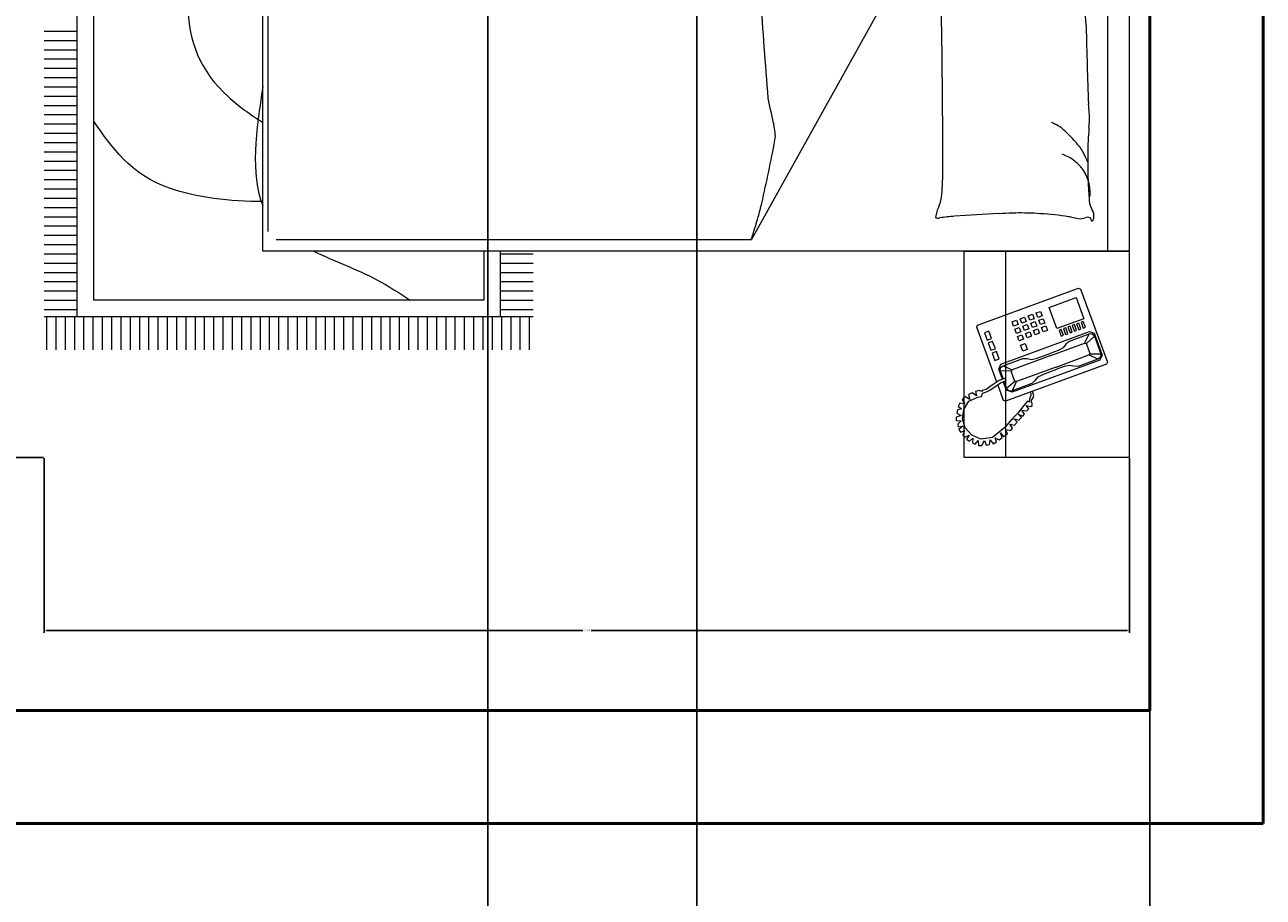
# Model space of a CAD drawing. Units: inches. Extents: x 338 to 1188, y -996 to 127.
# Tile 10 of 15: x 859 to 957, y -622 to -552. Entities that reach past the tile are written whole.
import ezdxf

# ---------------------------------------------------------------- set-up
doc = ezdxf.new("R2010")
doc.units = ezdxf.units.IN
doc.header["$MEASUREMENT"] = 0
doc.layers.add('A-ANNO-DIMS', color=5, linetype='Continuous', lineweight=18)
doc.layers.add('wall', color=1, linetype='Continuous', lineweight=50)
doc.layers.add('furniture', color=50, linetype='Continuous', lineweight=13, transparency=0.8)
doc.styles.add('DIM_FONT', font='SIMPLEX.shx', dxfattribs={"width": 0.8})
doc.styles.get("Standard").update_dxf_attribs({"font": 'arial.ttf'})
doc.dimstyles.get("Standard").update_dxf_attribs({"dimtxt": 0.18, "dimasz": 0.18, "dimexe": 0.18, "dimexo": 0.0625, "dimgap": 0.09, "dimtad": 0, "dimtih": 1, "dimtoh": 1, "dimdec": 1, "dimzin": 0, "dimdsep": 46, "dimlunit": 4, "dimtxsty": 'Standard', "dimcen": 0.09, "dimadec": 0, "dimazin": 0, "dimtfac": 1, "dimtdec": 1, "dimtofl": 0, "dimtmove": 0, "dimatfit": 3, "dimfxl": 1, "dimtolj": 1, "dimtzin": 0, "dimarcsym": 0})

# ---------------------------------------------------------------- blocks, each defined once
blk = doc.blocks.new('A$C4F634EDD')
for p, q in [((0.5, 2.6295), (2.3, 2.6295)), ((2.3, 2.6295), (2.3, 0.5295)), ((2.3, 2.6295), (2.8, 2.6295)), ((2.3, 2.2295), (2.3, 2.6295)), ((2.8, 2.6295), (2.8, 2.2295)), ((0.5, 2.5771), (2.3, 2.5771)), ((2.392, 2.5115), (2.5692, 2.5765)), ((2.4985, 2.5445), (2.5516, 2.564)), ((2.5062, 2.5454), (2.5487, 2.561)), ((2.5483, 2.5347), (2.5487, 2.561)), ((2.5487, 2.561), (2.5571, 2.56)), ((2.5615, 2.5536), (2.5514, 2.5318)), ((2.5516, 2.564), (2.5637, 2.5584)), ((2.5571, 2.56), (2.5615, 2.5536)), ((2.5615, 2.5536), (2.5791, 2.5058)), ((2.5637, 2.5584), (2.6418, 2.3458)), ((2.5692, 2.5765), (2.574, 2.5743)), ((2.574, 2.5743), (2.6638, 2.3298)), ((2.4842, 2.5232), (2.47, 2.518)), ((2.4862, 2.5179), (2.4842, 2.5232)), ((2.4946, 2.5331), (2.4985, 2.5445)), ((2.5734, 2.3187), (2.4946, 2.5331)), ((2.5062, 2.5454), (2.5004, 2.5392)), ((2.5004, 2.5392), (2.5013, 2.5315)), ((2.5013, 2.5315), (2.5188, 2.4836)), ((2.5013, 2.5315), (2.5231, 2.5214)), ((2.5235, 2.5256), (2.5062, 2.5454)), ((2.5231, 2.5214), (2.5235, 2.5256)), ((2.5483, 2.5347), (2.5235, 2.5256)), ((2.5514, 2.5318), (2.5483, 2.5347)), ((2.5807, 2.4521), (2.5514, 2.5318)), ((2.3898, 2.5066), (2.392, 2.5115)), ((2.4795, 2.2621), (2.3898, 2.5066)), ((2.412, 2.5007), (2.4634, 2.5196)), ((2.4361, 2.4352), (2.412, 2.5007)), ((2.4634, 2.5196), (2.4875, 2.454)), ((2.47, 2.518), (2.472, 2.5127)), ((2.472, 2.5127), (2.4862, 2.5179)), ((2.4881, 2.5126), (2.4739, 2.5074)), ((2.4739, 2.5074), (2.4759, 2.502)), ((2.4759, 2.502), (2.4901, 2.5073)), ((2.492, 2.5019), (2.4778, 2.4967)), ((2.4778, 2.4967), (2.4798, 2.4914)), ((2.4798, 2.4914), (2.494, 2.4966)), ((2.4901, 2.5073), (2.4881, 2.5126)), ((2.494, 2.4966), (2.492, 2.5019)), ((2.5523, 2.4417), (2.5231, 2.5214)), ((2.5788, 2.4956), (2.5767, 2.4848)), ((2.5791, 2.5058), (2.5788, 2.4956)), ((2.4959, 2.4913), (2.4817, 2.4861)), ((2.4817, 2.4861), (2.4837, 2.4808)), ((2.4837, 2.4808), (2.4979, 2.486)), ((2.4998, 2.4807), (2.4856, 2.4755)), ((2.4856, 2.4755), (2.4876, 2.4702)), ((2.4876, 2.4702), (2.5018, 2.4754)), ((2.5037, 2.47), (2.4895, 2.4648)), ((2.4895, 2.4648), (2.4915, 2.4595)), ((2.4915, 2.4595), (2.5057, 2.4647)), ((2.4979, 2.486), (2.4959, 2.4913)), ((2.5018, 2.4754), (2.4998, 2.4807)), ((2.5057, 2.4647), (2.5037, 2.47)), ((2.5188, 2.4836), (2.5256, 2.4761)), ((2.5256, 2.4761), (2.5342, 2.4692)), ((2.5342, 2.4692), (2.5405, 2.4574)), ((2.5767, 2.4848), (2.5795, 2.4717)), ((2.5795, 2.4717), (2.586, 2.454)), ((2.4875, 2.454), (2.4361, 2.4352)), ((2.4811, 2.4276), (2.4917, 2.4315)), ((2.4917, 2.4315), (2.4956, 2.4208)), ((2.5405, 2.4574), (2.547, 2.4397)), ((2.5594, 2.4061), (2.547, 2.4397)), ((2.5523, 2.4417), (2.5875, 2.346)), ((2.5807, 2.4521), (2.6158, 2.3564)), ((2.5984, 2.4204), (2.586, 2.454)), ((2.4457, 2.4146), (2.4563, 2.4185)), ((2.4496, 2.4039), (2.4457, 2.4146)), ((2.4602, 2.4078), (2.4496, 2.4039)), ((2.4563, 2.4185), (2.4602, 2.4078)), ((2.4634, 2.4211), (2.474, 2.425)), ((2.4673, 2.4104), (2.4634, 2.4211)), ((2.4779, 2.4143), (2.4673, 2.4104)), ((2.4706, 2.4016), (2.4812, 2.4055)), ((2.4745, 2.3909), (2.4706, 2.4016)), ((2.474, 2.425), (2.4779, 2.4143)), ((2.485, 2.4169), (2.4811, 2.4276)), ((2.4812, 2.4055), (2.4851, 2.3949)), ((2.4956, 2.4208), (2.485, 2.4169)), ((2.4883, 2.4081), (2.4989, 2.412)), ((2.4922, 2.3975), (2.4883, 2.4081)), ((2.5028, 2.4014), (2.4922, 2.3975)), ((2.4989, 2.412), (2.5028, 2.4014)), ((2.5622, 2.393), (2.5594, 2.4061)), ((2.6047, 2.4086), (2.5984, 2.4204)), ((2.6133, 2.4017), (2.6047, 2.4086)), ((2.6201, 2.3941), (2.6133, 2.4017)), ((2.4528, 2.3951), (2.4635, 2.399)), ((2.4567, 2.3844), (2.4528, 2.3951)), ((2.4674, 2.3883), (2.4567, 2.3844)), ((2.46, 2.3756), (2.4706, 2.3795)), ((2.4639, 2.365), (2.46, 2.3756)), ((2.4635, 2.399), (2.4674, 2.3883)), ((2.4706, 2.3795), (2.4745, 2.3689)), ((2.4851, 2.3949), (2.4745, 2.3909)), ((2.4777, 2.3821), (2.4883, 2.386)), ((2.4816, 2.3715), (2.4777, 2.3821)), ((2.4922, 2.3754), (2.4816, 2.3715)), ((2.4883, 2.386), (2.4922, 2.3754)), ((2.4954, 2.3886), (2.5061, 2.3925)), ((2.4993, 2.378), (2.4954, 2.3886)), ((2.51, 2.3819), (2.4993, 2.378)), ((2.5026, 2.3691), (2.5132, 2.373)), ((2.5061, 2.3925), (2.51, 2.3819)), ((2.5132, 2.373), (2.5171, 2.3624)), ((2.5238, 2.3769), (2.538, 2.3821)), ((2.5277, 2.3663), (2.5238, 2.3769)), ((2.5419, 2.3715), (2.5277, 2.3663)), ((2.538, 2.3821), (2.5419, 2.3715)), ((2.5598, 2.372), (2.5601, 2.3822)), ((2.5774, 2.3242), (2.5598, 2.372)), ((2.5601, 2.3822), (2.5622, 2.393)), ((2.6376, 2.3463), (2.6201, 2.3941)), ((2.6499, 2.3979), (2.6397, 2.3953)), ((2.6417, 2.39), (2.6488, 2.391)), ((2.6488, 2.391), (2.6538, 2.3895)), ((2.6551, 2.397), (2.6499, 2.3979)), ((2.6538, 2.3895), (2.6596, 2.388)), ((2.6627, 2.392), (2.6551, 2.397)), ((2.6596, 2.388), (2.6626, 2.3867)), ((2.6626, 2.3867), (2.6662, 2.388)), ((2.6692, 2.394), (2.6627, 2.392)), ((2.6662, 2.388), (2.6632, 2.3828)), ((2.6632, 2.3828), (2.6736, 2.3744)), ((2.6736, 2.3944), (2.6692, 2.394)), ((2.6765, 2.391), (2.6736, 2.3944)), ((2.6736, 2.3744), (2.6922, 2.3593)), ((2.6742, 2.3795), (2.6765, 2.391)), ((2.6824, 2.3858), (2.6742, 2.3795)), ((2.6873, 2.3815), (2.6824, 2.3858)), ((2.6853, 2.369), (2.6873, 2.3815)), ((2.6946, 2.376), (2.6853, 2.369)), ((2.6995, 2.3713), (2.6946, 2.376)), ((2.695, 2.3603), (2.6995, 2.3713)), ((2.4745, 2.3689), (2.4639, 2.365)), ((2.4672, 2.3561), (2.4778, 2.36)), ((2.4711, 2.3455), (2.4672, 2.3561)), ((2.4817, 2.3494), (2.4711, 2.3455)), ((2.4778, 2.36), (2.4817, 2.3494)), ((2.4849, 2.3626), (2.4955, 2.3665)), ((2.4888, 2.352), (2.4849, 2.3626)), ((2.4994, 2.3559), (2.4888, 2.352)), ((2.4955, 2.3665), (2.4994, 2.3559)), ((2.5065, 2.3585), (2.5026, 2.3691)), ((2.5171, 2.3624), (2.5065, 2.3585)), ((2.5774, 2.3242), (2.5875, 2.346)), ((2.5875, 2.346), (2.5905, 2.3431)), ((2.5905, 2.3431), (2.5901, 2.3168)), ((2.6154, 2.3522), (2.5905, 2.3431)), ((2.6158, 2.3564), (2.6154, 2.3522)), ((2.6154, 2.3522), (2.6327, 2.3324)), ((2.6376, 2.3463), (2.6158, 2.3564)), ((2.6418, 2.3458), (2.6369, 2.332)), ((2.6385, 2.3386), (2.6376, 2.3463)), ((2.6922, 2.3593), (2.7051, 2.3473)), ((2.7031, 2.3682), (2.695, 2.3603)), ((2.7096, 2.3616), (2.7031, 2.3682)), ((2.7051, 2.3473), (2.7079, 2.3475)), ((2.7062, 2.351), (2.7096, 2.3616)), ((2.7147, 2.3578), (2.7062, 2.351)), ((2.7079, 2.3475), (2.7079, 2.3443)), ((2.7079, 2.3443), (2.727, 2.3277)), ((2.7214, 2.3517), (2.7147, 2.3578)), ((2.7196, 2.34), (2.7214, 2.3517)), ((2.7286, 2.3466), (2.7196, 2.34)), ((2.7346, 2.3423), (2.7286, 2.3466)), ((2.732, 2.3295), (2.7346, 2.3423)), ((2.8, 2.3301), (2.3, 2.3301)), ((2.561, 2.3141), (2.5433, 2.3076)), ((2.5649, 2.3035), (2.561, 2.3141)), ((2.5855, 2.3131), (2.5734, 2.3187)), ((2.5818, 2.3178), (2.5774, 2.3242)), ((2.5901, 2.3168), (2.5818, 2.3178)), ((2.6104, 2.3222), (2.5855, 2.3131)), ((2.5901, 2.3168), (2.6097, 2.324)), ((2.613, 2.3312), (2.6077, 2.3293)), ((2.6077, 2.3293), (2.6135, 2.3141)), ((2.6192, 2.3174), (2.613, 2.3312)), ((2.6135, 2.3141), (2.6244, 2.2977)), ((2.6153, 2.3261), (2.6327, 2.3324)), ((2.6369, 2.332), (2.6161, 2.3243)), ((2.626, 2.3069), (2.6192, 2.3174)), ((2.6616, 2.3249), (2.6234, 2.3109)), ((2.6327, 2.3324), (2.6385, 2.3386)), ((2.6638, 2.3298), (2.6616, 2.3249)), ((2.727, 2.3277), (2.7512, 2.2983)), ((2.7423, 2.3345), (2.732, 2.3295)), ((2.7406, 2.3172), (2.7495, 2.325)), ((2.7519, 2.3218), (2.7406, 2.3172)), ((2.7495, 2.325), (2.7423, 2.3345)), ((2.7575, 2.3144), (2.7519, 2.3218)), ((2.7526, 2.3045), (2.7575, 2.3144)), ((2.6172, 2.3086), (2.4844, 2.2599)), ((2.5114, 2.2959), (2.4936, 2.2894)), ((2.4936, 2.2894), (2.4976, 2.2788)), ((2.4976, 2.2788), (2.5153, 2.2853)), ((2.5153, 2.2853), (2.5114, 2.2959)), ((2.5362, 2.305), (2.5185, 2.2985)), ((2.5185, 2.2985), (2.5224, 2.2879)), ((2.5224, 2.2879), (2.5401, 2.2944)), ((2.5401, 2.2944), (2.5362, 2.305)), ((2.5433, 2.3076), (2.5472, 2.297)), ((2.5472, 2.297), (2.5649, 2.3035)), ((2.6244, 2.2977), (2.6349, 2.2825)), ((2.6365, 2.2916), (2.626, 2.3069)), ((2.6349, 2.2825), (2.638, 2.273)), ((2.6407, 2.2834), (2.6365, 2.2916)), ((2.6438, 2.2739), (2.6407, 2.2834)), ((2.7512, 2.2983), (2.756, 2.2695)), ((2.7622, 2.308), (2.7526, 2.3045)), ((2.7574, 2.2924), (2.7673, 2.2997)), ((2.7687, 2.2905), (2.7574, 2.2924)), ((2.7587, 2.279), (2.7699, 2.2828)), ((2.7673, 2.2997), (2.7622, 2.308)), ((2.7699, 2.2828), (2.7687, 2.2905)), ((2.4844, 2.2599), (2.4795, 2.2621)), ((2.6399, 2.2712), (2.6374, 2.2659)), ((2.6374, 2.2659), (2.6398, 2.257)), ((2.638, 2.273), (2.6399, 2.2712)), ((2.6398, 2.257), (2.6509, 2.259)), ((2.6509, 2.259), (2.6431, 2.2492)), ((2.6519, 2.2716), (2.6438, 2.2739)), ((2.6535, 2.2628), (2.6519, 2.2716)), ((2.6636, 2.2409), (2.6535, 2.2628)), ((2.756, 2.2695), (2.7459, 2.2483)), ((2.7708, 2.2725), (2.7587, 2.279)), ((2.759, 2.2637), (2.7706, 2.2643)), ((2.7676, 2.2559), (2.759, 2.2637)), ((2.7645, 2.2498), (2.7676, 2.2559)), ((2.7706, 2.2643), (2.7708, 2.2725)), ((2.8, 2.2295), (2.3, 2.2295)), ((2.6431, 2.2492), (2.6473, 2.2398)), ((2.6473, 2.2398), (2.6592, 2.2429)), ((2.6592, 2.2429), (2.6521, 2.2314)), ((2.6521, 2.2314), (2.6598, 2.2248)), ((2.6598, 2.2248), (2.6697, 2.2309)), ((2.6836, 2.2287), (2.6636, 2.2409)), ((2.6697, 2.2309), (2.6684, 2.219)), ((2.6761, 2.2145), (2.6821, 2.2237)), ((2.6821, 2.2237), (2.6843, 2.2135)), ((2.7063, 2.2256), (2.6836, 2.2287)), ((2.6927, 2.2117), (2.6986, 2.222)), ((2.6986, 2.222), (2.7019, 2.2098)), ((2.7284, 2.2317), (2.7063, 2.2256)), ((2.7102, 2.2104), (2.7113, 2.2218)), ((2.7113, 2.2218), (2.7192, 2.2137)), ((2.7255, 2.2152), (2.7242, 2.2265)), ((2.7242, 2.2265), (2.7324, 2.2165)), ((2.7459, 2.2483), (2.7284, 2.2317)), ((2.7386, 2.2208), (2.7354, 2.2306)), ((2.7354, 2.2306), (2.7462, 2.2264)), ((2.7509, 2.2314), (2.7459, 2.2418)), ((2.7459, 2.2418), (2.7568, 2.2352)), ((2.7462, 2.2264), (2.7509, 2.2314)), ((2.7529, 2.2505), (2.7645, 2.2498)), ((2.7607, 2.2424), (2.7529, 2.2505)), ((2.7568, 2.2352), (2.7607, 2.2424)), ((2.6684, 2.219), (2.6761, 2.2145)), ((2.6843, 2.2135), (2.6927, 2.2117)), ((2.7019, 2.2098), (2.7102, 2.2104)), ((2.7192, 2.2137), (2.7255, 2.2152)), ((2.7324, 2.2165), (2.7386, 2.2208)), ((1.5035, 2.141), (2.2716, 1.7136)), ((2.2716, 0.5617), (2.2716, 1.7136)), ((2.3061, 1.1052), (2.3061, 1.1852)), ((2.3286, 1.1052), (2.3286, 1.1852)), ((2.3511, 1.1052), (2.3511, 1.1852)), ((2.3736, 1.1052), (2.3736, 1.1852)), ((2.3961, 1.1052), (2.3961, 1.1852)), ((2.4186, 1.1052), (2.4186, 1.1852)), ((2.4411, 1.1052), (2.4411, 1.1852)), ((2.4588, 1.1852), (2.4588, 0)), ((2.4588, 1.1753), (2.5388, 1.1753)), ((2.4588, 1.1528), (2.5388, 1.1528)), ((2.4588, 1.1303), (2.5388, 1.1303)), ((2.3, 1.1052), (2.4588, 1.1052)), ((2.4588, 1.1078), (2.5388, 1.1078)), ((2.4588, 1.0853), (2.5388, 1.0853)), ((2.3, 1.0652), (2.4188, 1.0652)), ((2.4188, 1.0652), (2.4188, 0.12)), ((2.4588, 1.0628), (2.5388, 1.0628)), ((2.4588, 1.0403), (2.5388, 1.0403)), ((2.4588, 1.0178), (2.5388, 1.0178)), ((2.4588, 0.9953), (2.5388, 0.9953)), ((2.4588, 0.9728), (2.5388, 0.9728)), ((2.4588, 0.9503), (2.5388, 0.9503)), ((2.4588, 0.9278), (2.5388, 0.9278)), ((2.4588, 0.9053), (2.5388, 0.9053)), ((2.4588, 0.8828), (2.5388, 0.8828)), ((2.4588, 0.8603), (2.5388, 0.8603)), ((2.4588, 0.8378), (2.5388, 0.8378)), ((2.4588, 0.8153), (2.5388, 0.8153)), ((2.4588, 0.7928), (2.5388, 0.7928)), ((2.4588, 0.7703), (2.5388, 0.7703)), ((2.4588, 0.7478), (2.5388, 0.7478)), ((2.4588, 0.7253), (2.5388, 0.7253)), ((2.4588, 0.7028), (2.5388, 0.7028)), ((2.4588, 0.6803), (2.5388, 0.6803)), ((2.4588, 0.6578), (2.5388, 0.6578)), ((2.4588, 0.6353), (2.5388, 0.6353)), ((2.4588, 0.6128), (2.5388, 0.6128)), ((2.4588, 0.5903), (2.5388, 0.5903)), ((0.5458, 0.5417), (2.2516, 0.5417)), ((2.4588, 0.5678), (2.5388, 0.5678)), ((2.4588, 0.5453), (2.5388, 0.5453)), ((2.3, 0.5295), (0.5, 0.5295)), ((2.4588, 0.5228), (2.5388, 0.5228)), ((2.4588, 0.5003), (2.5388, 0.5003)), ((2.4588, 0.4778), (2.5388, 0.4778)), ((2.4588, 0.4553), (2.5388, 0.4553)), ((2.4588, 0.4328), (2.5388, 0.4328)), ((2.4588, 0.4103), (2.5388, 0.4103)), ((2.4588, 0.3878), (2.5388, 0.3878)), ((2.4588, 0.3653), (2.5388, 0.3653)), ((2.4588, 0.3428), (2.5388, 0.3428)), ((2.4588, 0.3203), (2.5388, 0.3203)), ((2.4588, 0.2978), (2.5388, 0.2978)), ((2.4588, 0.2753), (2.5388, 0.2753)), ((2.4588, 0.2528), (2.5388, 0.2528)), ((2.4588, 0.2303), (2.5388, 0.2303)), ((2.4588, 0.2078), (2.5388, 0.2078)), ((2.4588, 0.1853), (2.5388, 0.1853)), ((2.4588, 0.1628), (2.5388, 0.1628)), ((2.4588, 0.1403), (2.5388, 0.1403)), ((2.4188, 0.12), (0.3786, 0.12)), ((2.4588, 0.1178), (2.5388, 0.1178)), ((2.4588, 0.0953), (2.5388, 0.0953)), ((2.4588, 0.08), (0.3386, 0.08)), ((1.7661, 0), (1.7661, 0.08)), ((1.7886, 0), (1.7886, 0.08)), ((1.8111, 0), (1.8111, 0.08)), ((1.8336, 0), (1.8336, 0.08)), ((1.8561, 0), (1.8561, 0.08)), ((1.8786, 0), (1.8786, 0.08)), ((1.9011, 0), (1.9011, 0.08)), ((1.9236, 0), (1.9236, 0.08)), ((1.9461, 0), (1.9461, 0.08)), ((1.9686, 0), (1.9686, 0.08)), ((1.9911, 0), (1.9911, 0.08)), ((2.0136, 0), (2.0136, 0.08)), ((2.0361, 0), (2.0361, 0.08)), ((2.0586, 0), (2.0586, 0.08)), ((2.0811, 0), (2.0811, 0.08)), ((2.1036, 0), (2.1036, 0.08)), ((2.1261, 0), (2.1261, 0.08)), ((2.1486, 0), (2.1486, 0.08)), ((2.1711, 0), (2.1711, 0.08)), ((2.1936, 0), (2.1936, 0.08)), ((2.2161, 0), (2.2161, 0.08)), ((2.2386, 0), (2.2386, 0.08)), ((2.2611, 0), (2.2611, 0.08)), ((2.2836, 0), (2.2836, 0.08)), ((2.3061, 0), (2.3061, 0.08)), ((2.3286, 0), (2.3286, 0.08)), ((2.3511, 0), (2.3511, 0.08)), ((2.3736, 0), (2.3736, 0.08)), ((2.3961, 0), (2.3961, 0.08)), ((2.4186, 0), (2.4186, 0.08)), ((2.4411, 0), (2.4411, 0.08)), ((2.4588, 0.0728), (2.5388, 0.0728)), ((2.4588, 0.0503), (2.5388, 0.0503)), ((2.4588, 0.0278), (2.5388, 0.0278)), ((2.4588, 0.0053), (2.5388, 0.0053))]:
    blk.add_line(p, q)
for centre, radius, start, end in [((1.6443, 3.5682), 1.049, 270, 276.0867), ((1.4785, 15.4878), 12.9656, 271.22425, 272.05324), ((1.97, 2.3805), 0.1524, 92.5386, 100.1899), ((1.9761, 2.2433), 0.2897, 85.1982, 92.5386), ((2.0734, 3.4021), 0.8732, 265.1982, 269.4243), ((2.1674, 2.3102), 0.234, 110.8603, 117.2396), ((2.0797, 4.0232), 1.4943, 269.4243, 271.9079), ((2.1588, 2.4357), 0.0992, 105.9352, 126.0864), ((2.1021, 3.3501), 0.8208, 271.9079, 275.2592), ((2.1588, 2.4357), 0.0992, 85.7841, 105.9352), ((2.1724, 2.5864), 0.0539, 275.2592, 300.6513), ((2.2146, 2.5152), 0.0289, 85.6975, 120.6513), ((2.2149, 2.519), 0.0251, 68.2117, 85.6975), ((2.2331, 2.5288), 0.0156, 158.0096, 201.421), ((2.2226, 2.533), 0.00428, 78.1069, 158.0096), ((2.1881, 2.5111), 0.0328, 351.8665, 21.421), ((2.224, 2.5395), 0.00232, 258.1069, 19.564), ((2.2229, 2.5391), 0.00342, 19.564, 68.2117), ((2.291, 2.2032), 0.3916, 128.3886, 133.8115), ((2.0954, 2.45), 0.0768, 117.2396, 128.3886), ((2.1588, 2.4357), 0.0992, 143.8234, 161.5603), ((2.1588, 2.4357), 0.0992, 126.0864, 143.8234), ((1.977, 2.5413), 0.246, 347.8905, 351.8665), ((2.0391, 2.4341), 0.0493, 140.9651, 151.6832), ((2.1757, 2.3233), 0.2252, 133.8115, 140.9651), ((3.1198, 2.3525), 0.9131, 172.3191, 176.6313), ((2.4114, 2.448), 0.1983, 167.8905, 172.3191), ((2.1719, 2.3625), 0.2002, 151.6832, 156.9972), ((2.8858, 2.3663), 0.6787, 176.6313, 181.6331), ((3.5721, 2.3859), 1.3652, 181.6331, 183.055), ((15.8249, 3.0398), 13.6356, 183.05496, 183.50486), ((2.5355, 2.2258), 0.3212, 183.5049, 189.9984), ((2.1093, -19.8405), 22.0183, 90.37908, 91.01965), ((2.0605, -3.5404), 5.7185, 89.7135, 90.9704), ((2.0833, 1.0141), 1.164, 86.426, 89.7135), ((2.1467, 2.0302), 0.1459, 77.131, 86.426), ((2.1691, 2.1283), 0.0453, 62.7159, 77.131), ((2.2251, 2.2367), 0.0767, 242.7159, 253.7788), ((2.2281, 2.247), 0.0875, 253.7788, 262.8796), ((2.2001, 2.1667), 0.0193, 343.3022, 9.9984), ((2.2174, 2.1615), 0.00132, 262.8796, 343.3022), ((2.0378, 1.5789), 0.1942, 97.7304, 103.1904), ((2.0195, 1.7137), 0.0581, 79.2724, 97.7304), ((0.6102, 18.0525), 16.3521, 273.75703, 274.62393), ((1.4194, 4.2174), 2.5158, 281.6741, 283.1904), ((1.2737, -2.2227), 4.0646, 77.0745, 79.2724), ((2.0359, 1.0981), 0.6574, 74.0648, 77.0745), ((1.7125, -0.0344), 1.8351, 72.2636, 74.0648)]:
    blk.add_arc(centre, radius, start, end)
for points, knots in [([(2.3, 0.6535), (2.3236, 0.7026), (2.3554, 0.7914), (2.4015, 0.8608), (2.4188, 0.8868)], [1893.525221, 1893.525221, 1893.525221, 1893.525221, 2051.902476, 2146.74457, 2146.74457, 2146.74457, 2146.74457]), ([(1.2016, 0.5295), (1.2892, 0.479), (1.5144, 0.3684), (1.8265, 0.2994), (1.9681, 0.4992), (1.9875, 0.5295)], [936.534237, 936.534237, 936.534237, 936.534237, 1243.285375, 1683.261222, 1758.254386, 1758.254386, 1758.254386, 1758.254386]), ([(2.1796, 0.5295), (2.1798, 0.4519), (2.1548, 0.2369), (2.0487, 0.164), (1.9846, 0.12)], [2202.034493, 2202.034493, 2202.034493, 2202.034493, 2357.807635, 2594.446174, 2594.446174, 2594.446174, 2594.446174])]:
    blk.add_open_spline(points, degree=3, knots=knots)
blk.add_open_spline([(1.9003, 0.5295), (2.0065, 0.514), (2.1132, 0.4978), (2.1894, 0.5295)], degree=3)
at = {"style": 'DIM_FONT', "width": 0.8, "flags": 9}
for tag, p in [('YSIZE', (0.5, 2.6295)), ('XSIZE', (0.5, 2.6295)), ('XSIZE', (2.2985, 2.6295)), ('YSIZE', (2.2985, 2.6295))]:
    blk.add_attdef(tag, p, '', height=0.0005, dxfattribs=at)
blk = doc.blocks.new('*D19')
at = {"layer": 'A-ANNO-DIMS', "color": 0, "lineweight": -2, "transparency": 16777216}
for p, q in [((860.056, -494.839), (846.17, -494.839)), ((846.35, -495.019), (846.35, -540.551)), ((846.35, -586.447), (846.35, -540.915)), ((860.056, -586.627), (846.17, -586.627))]:
    blk.add_line(p, q, dxfattribs=at)
at = {"layer": 'A-ANNO-DIMS', "color": 0, "transparency": 16777216}
for points in [[(846.32, -495.019), (846.38, -495.019), (846.35, -494.839)], [(846.32, -586.447), (846.38, -586.447), (846.35, -586.627)]]:
    blk.add_solid(points, dxfattribs=at)
at = {"layer": 'Defpoints', "color": 0, "transparency": 16777216}
for p in [(860.118, -494.839), (846.35, -586.627), (860.118, -586.627)]:
    blk.add_point(p, dxfattribs=at)
at = {"layer": 'A-ANNO-DIMS', "color": 0, "transparency": 16777216, "insert": (846.35, -540.733), "char_height": 0.18, "attachment_point": 5}
blk.add_mtext('\\A1;BED 7\'-8"', dxfattribs=at)
blk = doc.blocks.new('*D20')
at = {"layer": 'A-ANNO-DIMS', "color": 0, "lineweight": -2, "transparency": 16777216}
for p, q in [((860.118, -586.689), (860.118, -600.575)), ((946.333, -586.689), (946.333, -600.575)), ((860.298, -600.395), (902.897, -600.395)), ((946.153, -600.395), (903.554, -600.395))]:
    blk.add_line(p, q, dxfattribs=at)
at = {"layer": 'A-ANNO-DIMS', "color": 0, "transparency": 16777216}
for points in [[(860.298, -600.365), (860.298, -600.425), (860.118, -600.395)], [(946.153, -600.365), (946.153, -600.425), (946.333, -600.395)]]:
    blk.add_solid(points, dxfattribs=at)
at = {"layer": 'Defpoints', "color": 0, "transparency": 16777216}
for p in [(860.118, -586.627), (946.333, -586.627), (946.333, -600.395)]:
    blk.add_point(p, dxfattribs=at)
at = {"layer": 'A-ANNO-DIMS', "color": 0, "transparency": 16777216, "insert": (903.226, -600.395), "char_height": 0.18, "attachment_point": 5}
blk.add_mtext('\\A1;7\'-2"', dxfattribs=at)
blk = doc.blocks.new('*D27')
at = {"layer": 'A-ANNO-DIMS', "color": 0, "lineweight": -2, "transparency": 16777216}
for p, q in [((911.963, -297.796), (911.963, -968.856)), ((947.963, -297.796), (947.963, -968.856)), ((912.143, -968.676), (929.634, -968.676)), ((947.783, -968.676), (930.292, -968.676))]:
    blk.add_line(p, q, dxfattribs=at)
at = {"layer": 'A-ANNO-DIMS', "color": 0, "transparency": 16777216}
for points in [[(912.143, -968.646), (912.143, -968.706), (911.963, -968.676)], [(947.783, -968.646), (947.783, -968.706), (947.963, -968.676)]]:
    blk.add_solid(points, dxfattribs=at)
at = {"layer": 'Defpoints', "color": 0, "transparency": 16777216}
for p in [(911.963, -297.733), (947.963, -297.733), (947.963, -968.676)]:
    blk.add_point(p, dxfattribs=at)
at = {"layer": 'A-ANNO-DIMS', "color": 0, "transparency": 16777216, "insert": (929.963, -968.676), "char_height": 0.18, "attachment_point": 5}
blk.add_mtext('\\A1;3\'-0"', dxfattribs=at)
blk = doc.blocks.new('*D28')
at = {"layer": 'A-ANNO-DIMS', "color": 0, "lineweight": -2, "transparency": 16777216}
for p, q in [((803.963, -265.796), (803.963, -968.856)), ((947.963, -297.796), (947.963, -968.856)), ((804.143, -968.676), (875.573, -968.676)), ((947.783, -968.676), (876.354, -968.676))]:
    blk.add_line(p, q, dxfattribs=at)
at = {"layer": 'A-ANNO-DIMS', "color": 0, "transparency": 16777216}
for points in [[(804.143, -968.646), (804.143, -968.706), (803.963, -968.676)], [(947.783, -968.646), (947.783, -968.706), (947.963, -968.676)]]:
    blk.add_solid(points, dxfattribs=at)
at = {"layer": 'Defpoints', "color": 0, "transparency": 16777216}
for p in [(803.963, -265.733), (947.963, -297.733), (947.963, -968.676)]:
    blk.add_point(p, dxfattribs=at)
at = {"layer": 'A-ANNO-DIMS', "color": 0, "transparency": 16777216, "insert": (875.963, -968.676), "char_height": 0.18, "attachment_point": 5}
blk.add_mtext('\\A1;12\'-0"', dxfattribs=at)
blk = doc.blocks.new('*D43')
at = {"layer": 'A-ANNO-DIMS', "color": 0, "lineweight": -2, "transparency": 16777216}
for p, q in [((853.279, -53.934), (853.279, -968.856)), ((895.369, -53.934), (895.369, -968.856)), ((853.459, -968.676), (873.995, -968.676)), ((895.189, -968.676), (874.653, -968.676))]:
    blk.add_line(p, q, dxfattribs=at)
at = {"layer": 'A-ANNO-DIMS', "color": 0, "transparency": 16777216}
for points in [[(853.459, -968.646), (853.459, -968.706), (853.279, -968.676)], [(895.189, -968.646), (895.189, -968.706), (895.369, -968.676)]]:
    blk.add_solid(points, dxfattribs=at)
at = {"layer": 'Defpoints', "color": 0, "transparency": 16777216}
for p in [(853.279, -53.872), (895.369, -53.872), (895.369, -968.676)]:
    blk.add_point(p, dxfattribs=at)
at = {"layer": 'A-ANNO-DIMS', "color": 0, "transparency": 16777216, "insert": (874.324, -968.676), "char_height": 0.18, "attachment_point": 5}
blk.add_mtext('\\A1;3\'-6"', dxfattribs=at)
blk = doc.blocks.new('*D44')
at = {"layer": 'A-ANNO-DIMS', "color": 0, "lineweight": -2, "transparency": 16777216}
for p, q in [((895.369, -53.934), (895.369, -968.856)), ((947.963, -54.796), (947.963, -968.856)), ((895.549, -968.676), (921.124, -968.676)), ((947.783, -968.676), (922.209, -968.676))]:
    blk.add_line(p, q, dxfattribs=at)
at = {"layer": 'A-ANNO-DIMS', "color": 0, "transparency": 16777216}
for points in [[(895.549, -968.646), (895.549, -968.706), (895.369, -968.676)], [(947.783, -968.646), (947.783, -968.706), (947.963, -968.676)]]:
    blk.add_solid(points, dxfattribs=at)
at = {"layer": 'Defpoints', "color": 0, "transparency": 16777216}
for p in [(895.369, -53.872), (947.963, -54.733), (947.963, -968.676)]:
    blk.add_point(p, dxfattribs=at)
at = {"layer": 'A-ANNO-DIMS', "color": 0, "transparency": 16777216, "insert": (921.666, -968.676), "char_height": 0.18, "attachment_point": 5}
blk.add_mtext('\\A1;4\'-4 1/2"', dxfattribs=at)
blk = doc.blocks.new('*D47')
at = {"layer": 'A-ANNO-DIMS', "color": 0, "lineweight": -2, "transparency": 16777216}
for p, q in [((759.673, -755.171), (759.673, 67.247)), ((759.853, 67.067), (867.678, 67.067)), ((976.283, 67.067), (868.459, 67.067)), ((976.463, -755.171), (976.463, 67.247))]:
    blk.add_line(p, q, dxfattribs=at)
at = {"layer": 'A-ANNO-DIMS', "color": 0, "transparency": 16777216}
for points in [[(759.853, 67.097), (759.853, 67.037), (759.673, 67.067)], [(976.283, 67.097), (976.283, 67.037), (976.463, 67.067)]]:
    blk.add_solid(points, dxfattribs=at)
at = {"layer": 'Defpoints', "color": 0, "transparency": 16777216}
for p in [(976.463, 67.067), (759.673, -755.233), (976.463, -755.233)]:
    blk.add_point(p, dxfattribs=at)
at = {"layer": 'A-ANNO-DIMS', "color": 0, "transparency": 16777216, "insert": (868.068, 67.067), "char_height": 0.18, "attachment_point": 5}
blk.add_mtext('\\A1;18\'-1"', dxfattribs=at)

msp = doc.modelspace()

# ---------------------------------------------------------------- linework, layer by layer
at = {"layer": 'wall'}
for p, q in [((956.963, -15.733), (956.963, -615.733)), ((947.963, -474.733), (947.963, -606.733)), ((947.963, -606.733), (746.963, -606.733)), ((956.963, -615.733), (660.963, -615.733))]:
    msp.add_line(p, q, dxfattribs=at)

# ---------------------------------------------------------------- block references
at = {"layer": 'furniture', "xscale": 32.78135669785699, "yscale": 32.78135669785699, "zscale": 32.78135669785699, "rotation": 270}
msp.add_blockref('A$C4F634EDD', (860.118, -494.839), dxfattribs=at)

# ---------------------------------------------------------------- dimensions: what is measured, and where the dimension line sits
at = {"layer": 'A-ANNO-DIMS'}
for base, p1, p2, picture, middle in [((976.463, 67.067), (759.673, -755.233), (976.463, -755.233), '*D47', (868.068, 67.067)), ((895.369, -968.676), (853.279, -53.872), (895.369, -53.872), '*D43', (874.324, -968.676)), ((947.963, -968.676), (895.369, -53.872), (947.963, -54.733), '*D44', (921.666, -968.676)), ((947.963, -968.676), (803.963, -265.733), (947.963, -297.733), '*D28', (875.963, -968.676)), ((947.963, -968.676), (911.963, -297.733), (947.963, -297.733), '*D27', (929.963, -968.676)), ((946.333, -600.395), (860.118, -586.627), (946.333, -586.627), '*D20', (903.226, -600.395))]:
    dim = msp.add_linear_dim(base=base, p1=p1, p2=p2, dimstyle='Standard', override={"dimdec": 1, "dimlfac": 1, "dimrnd": 0, "dimzin": 1, "dimdsep": 46, "dimlunit": 4, "dimfrac": 2}, dxfattribs=at)
    dim.commit()
    dim.dimension.update_dxf_attribs({"geometry": picture, "text_midpoint": middle})
dim = msp.add_linear_dim(base=(846.35, -586.627), p1=(860.118, -494.839), p2=(860.118, -586.627), angle=270, text='BED <>', dimstyle='Standard', override={"dimdec": 1, "dimlfac": 1, "dimrnd": 0, "dimzin": 1, "dimdsep": 46, "dimlunit": 4, "dimfrac": 2}, dxfattribs=at)
dim.commit()
dim.dimension.update_dxf_attribs({"geometry": '*D19', "text_midpoint": (846.35, -540.733)})

doc.saveas('drawing.dxf')
